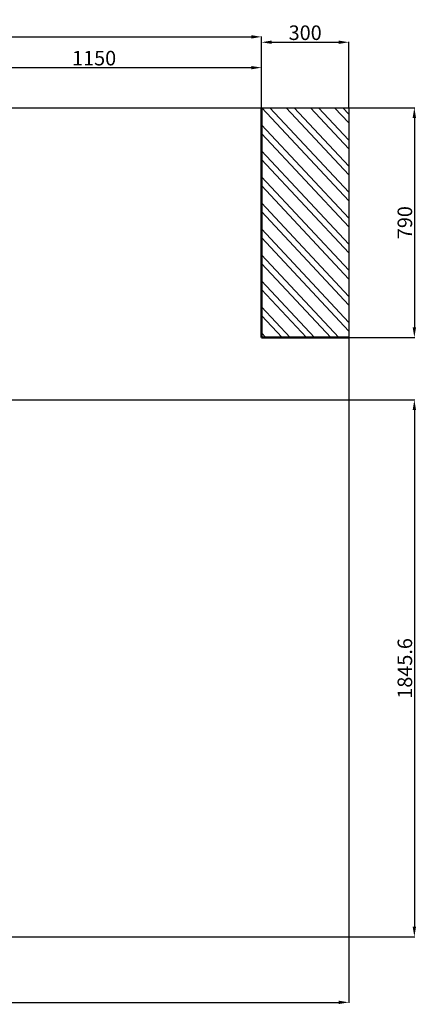
# Model space of a CAD drawing. Units: millimetres. Extents: x 407065 to 421840, y 1168257 to 1177792.
# Tile 2 of 17: x 410003 to 411365, y 1168454 to 1171838. Entities that reach past the tile are written whole.
import ezdxf

# ---------------------------------------------------------------- set-up
doc = ezdxf.new("R2010")
doc.units = ezdxf.units.MM
for name, color, linetype, lineweight in [('A-ANNO-DIMS', 6, 'Continuous', 18), ('A-FURN', 3, 'Continuous', 25), ('A-WALL', 7, 'Continuous', 50), ('A-WALL-PATT', 8, 'Continuous', 13)]:
    doc.layers.add(name, color=color, linetype=linetype, lineweight=lineweight)
doc.styles.get("Standard").update_dxf_attribs({"font": 'arial.ttf'})
doc.dimstyles.new('ISO-25', dxfattribs={"dimtxt": 50, "dimasz": 35, "dimexe": 1.25, "dimexo": 0.625, "dimtad": 1, "dimdec": 1, "dimtxsty": 'Standard', "dimcen": 35, "dimadec": 0, "dimazin": 0, "dimtfac": 1, "dimtdec": 1, "dimtmove": 0, "dimatfit": 3, "dimfxl": 1, "dimarcsym": 0})

# ---------------------------------------------------------------- blocks, each defined once
blk = doc.blocks.new('*D122')
at = {"layer": 'A-ANNO-DIMS', "color": 0, "lineweight": -2, "transparency": 16777216}
for p, q in [((409683.5, 1171673.4), (409683.5, 1171674.1)), ((409718.5, 1171672.8), (410798.5, 1171672.8)), ((410833.5, 1171673.4), (410833.5, 1171674.1))]:
    blk.add_line(p, q, dxfattribs=at)
at = {"layer": 'A-ANNO-DIMS', "color": 0, "transparency": 16777216}
for points in [[(409718.5, 1171678.6), (409718.5, 1171667), (409683.5, 1171672.8)], [(410798.5, 1171678.6), (410798.5, 1171667), (410833.5, 1171672.8)]]:
    blk.add_solid(points, dxfattribs=at)
at = {"layer": 'Defpoints', "color": 0, "transparency": 16777216}
for p in [(409683.5, 1171672.8), (410833.5, 1171672.8), (410833.5, 1171672.8)]:
    blk.add_point(p, dxfattribs=at)
at = {"layer": 'A-ANNO-DIMS', "color": 0, "transparency": 16777216, "insert": (410258.5, 1171699), "char_height": 50, "attachment_point": 5}
blk.add_mtext('1150', dxfattribs=at)
blk = doc.blocks.new('*D123')
at = {"layer": 'A-ANNO-DIMS', "color": 0, "lineweight": -2, "transparency": 16777216}
for p, q in [((408033.5, 1171744.1), (408033.5, 1171780)), ((408068.5, 1171778.7), (410798.5, 1171778.7)), ((410833.5, 1171744.1), (410833.5, 1171780))]:
    blk.add_line(p, q, dxfattribs=at)
at = {"layer": 'A-ANNO-DIMS', "color": 0, "transparency": 16777216}
for points in [[(408068.5, 1171784.5), (408068.5, 1171772.9), (408033.5, 1171778.7)], [(410798.5, 1171784.5), (410798.5, 1171772.9), (410833.5, 1171778.7)]]:
    blk.add_solid(points, dxfattribs=at)
at = {"layer": 'Defpoints', "color": 0, "transparency": 16777216}
for p in [(410833.5, 1171778.7), (408033.5, 1171743.5), (410833.5, 1171743.5)]:
    blk.add_point(p, dxfattribs=at)
at = {"layer": 'A-ANNO-DIMS', "color": 0, "transparency": 16777216, "insert": (409433.5, 1171804.9), "char_height": 50, "attachment_point": 5}
blk.add_mtext('2800', dxfattribs=at)
blk = doc.blocks.new('*D208')
at = {"layer": 'A-ANNO-DIMS', "color": 0, "lineweight": -2, "transparency": 16777216}
for p, q in [((407833.5, 1168684.6), (407833.5, 1168458.9)), ((411133.5, 1168684.6), (411133.5, 1168458.9)), ((407868.5, 1168460.2), (411098.5, 1168460.2))]:
    blk.add_line(p, q, dxfattribs=at)
at = {"layer": 'A-ANNO-DIMS', "color": 0, "transparency": 16777216}
for points in [[(407868.5, 1168466), (407868.5, 1168454.4), (407833.5, 1168460.2)], [(411098.5, 1168466), (411098.5, 1168454.4), (411133.5, 1168460.2)]]:
    blk.add_solid(points, dxfattribs=at)
at = {"layer": 'Defpoints', "color": 0, "transparency": 16777216}
for p in [(407833.5, 1168685.2), (411133.5, 1168685.2), (411133.5, 1168460.2)]:
    blk.add_point(p, dxfattribs=at)
at = {"layer": 'A-ANNO-DIMS', "color": 0, "transparency": 16777216, "insert": (409483.5, 1168486.4), "char_height": 50, "attachment_point": 5}
blk.add_mtext('3300', dxfattribs=at)
blk = doc.blocks.new('*D210')
at = {"layer": 'A-ANNO-DIMS', "color": 0, "lineweight": -2, "transparency": 16777216}
for p, q in [((410833.5, 1171535.8), (410833.5, 1171761.4)), ((410868.5, 1171760.2), (411098.5, 1171760.2)), ((411133.5, 1171535.8), (411133.5, 1171761.4))]:
    blk.add_line(p, q, dxfattribs=at)
at = {"layer": 'A-ANNO-DIMS', "color": 0, "transparency": 16777216}
for points in [[(410868.5, 1171766), (410868.5, 1171754.4), (410833.5, 1171760.2)], [(411098.5, 1171766), (411098.5, 1171754.4), (411133.5, 1171760.2)]]:
    blk.add_solid(points, dxfattribs=at)
at = {"layer": 'Defpoints', "color": 0, "transparency": 16777216}
for p in [(411133.5, 1171760.2), (410833.5, 1171535.2), (411133.5, 1171535.2)]:
    blk.add_point(p, dxfattribs=at)
at = {"layer": 'A-ANNO-DIMS', "color": 0, "transparency": 16777216, "insert": (410983.5, 1171786.4), "char_height": 50, "attachment_point": 5}
blk.add_mtext('300', dxfattribs=at)
blk = doc.blocks.new('*D211')
at = {"layer": 'A-ANNO-DIMS', "color": 0, "lineweight": -2, "transparency": 16777216}
for p, q in [((411134.2, 1171535.2), (411359.8, 1171535.2)), ((411358.5, 1171500.2), (411358.5, 1170780.2)), ((411134.2, 1170745.2), (411359.8, 1170745.2))]:
    blk.add_line(p, q, dxfattribs=at)
at = {"layer": 'A-ANNO-DIMS', "color": 0, "transparency": 16777216}
for points in [[(411352.7, 1171500.2), (411364.4, 1171500.2), (411358.5, 1171535.2)], [(411352.7, 1170780.2), (411364.4, 1170780.2), (411358.5, 1170745.2)]]:
    blk.add_solid(points, dxfattribs=at)
at = {"layer": 'Defpoints', "color": 0, "transparency": 16777216}
for p in [(411133.5, 1171535.2), (411133.5, 1170745.2), (411358.5, 1170745.2)]:
    blk.add_point(p, dxfattribs=at)
at = {"layer": 'A-ANNO-DIMS', "color": 0, "transparency": 16777216, "insert": (411332.4, 1171140.2), "char_height": 50, "attachment_point": 5, "rotation": 90}
blk.add_mtext('790', dxfattribs=at)
blk = doc.blocks.new('*D212')
at = {"layer": 'A-ANNO-DIMS', "color": 0, "lineweight": -2, "transparency": 16777216}
for p, q in [((409636.9, 1170530.8), (411359.8, 1170530.8)), ((411358.5, 1170495.8), (411358.5, 1168720.2)), ((409636.9, 1168685.2), (411359.8, 1168685.2))]:
    blk.add_line(p, q, dxfattribs=at)
at = {"layer": 'A-ANNO-DIMS', "color": 0, "transparency": 16777216}
for points in [[(411352.7, 1170495.8), (411364.4, 1170495.8), (411358.5, 1170530.8)], [(411352.7, 1168720.2), (411364.4, 1168720.2), (411358.5, 1168685.2)]]:
    blk.add_solid(points, dxfattribs=at)
at = {"layer": 'Defpoints', "color": 0, "transparency": 16777216}
for p in [(409636.3, 1170530.8), (409636.3, 1168685.2), (411358.5, 1168685.2)]:
    blk.add_point(p, dxfattribs=at)
at = {"layer": 'A-ANNO-DIMS', "color": 0, "transparency": 16777216, "insert": (411332.4, 1169608), "char_height": 50, "attachment_point": 5, "rotation": 90}
blk.add_mtext('1845.6', dxfattribs=at)

msp = doc.modelspace()

# ---------------------------------------------------------------- hatches: boundary and pattern name
at = {"layer": 'A-WALL-PATT'}
h = msp.add_hatch(dxfattribs=at)
h.set_pattern_fill('ANSI32', color=256, scale=6.4, angle=88)
h.set_pattern_definition([(133, (-5768.25, -464.17), (-44.5833217, -41.57462), []), (133, (-5767.245, -435.45), (-44.5833217, -41.57462), [])])
h.paths.add_polyline_path([(411133.5433, 1171535.1988), (410833.5433, 1171535.1988), (410833.5433, 1170745.1988), (411133.5433, 1170745.1988)])

# ---------------------------------------------------------------- linework, layer by layer
at = {"layer": 'A-FURN'}
for p, q in [((407833.5433, 1171535.1988), (411133.5433, 1171535.1988)), ((411133.5433, 1171535.1988), (411133.5433, 1168685.1988)), ((407833.5433, 1168685.1988), (411133.5433, 1168685.1988))]:
    msp.add_line(p, q, dxfattribs=at)
at = {"layer": 'A-WALL'}
for p, q in [((410833.5433, 1171535.1988), (410833.5433, 1170745.1988)), ((410833.5433, 1170745.1988), (411133.5433, 1170745.1988))]:
    msp.add_line(p, q, dxfattribs=at)

# ---------------------------------------------------------------- dimensions: what is measured, and where the dimension line sits
at = {"layer": 'A-ANNO-DIMS'}
for base, p1, p2, override, picture, middle in [((410833.5433, 1171778.705), (408033.5433, 1171743.4929), (410833.5433, 1171743.4929), {"dimclrd": 0, "dimclre": 0, "dimclrt": 0}, '*D123', (409433.5433, 1171804.8586)), ((411133.5433, 1171760.1988), (410833.5433, 1171535.1988), (411133.5433, 1171535.1988), {"dimdec": 0, "dimlfac": 1, "dimrnd": 0, "dimzin": 0, "dimdsep": 46, "dimlunit": 2}, '*D210', (410983.5433, 1171786.3695)), ((410833.5433, 1171672.8068), (409683.5433, 1171672.8068), (410833.5433, 1171672.8068), {"dimclrd": 0, "dimclre": 0, "dimclrt": 0}, '*D122', (410258.5433, 1171698.9605)), ((411133.5433, 1168460.1988), (407833.5433, 1168685.1988), (411133.5433, 1168685.1988), {"dimdec": 0, "dimlfac": 1, "dimrnd": 0, "dimzin": 0, "dimdsep": 46, "dimlunit": 2}, '*D208', (409483.5433, 1168486.3695))]:
    dim = msp.add_linear_dim(base=base, p1=p1, p2=p2, dimstyle='ISO-25', override=override, dxfattribs=at)
    dim.commit()
    dim.dimension.update_dxf_attribs({"geometry": picture, "text_midpoint": middle})
for base, p1, p2, override, picture, middle in [((411358.5433, 1170745.1988), (411133.5433, 1171535.1988), (411133.5433, 1170745.1988), {"dimdec": 0, "dimlfac": 1, "dimrnd": 0, "dimzin": 0, "dimdsep": 46, "dimlunit": 2}, '*D211', (411332.3896, 1171140.1988)), ((411358.5433, 1168685.1988), (409636.3246, 1170530.7673), (409636.3246, 1168685.1988), {"dimdec": 1, "dimlfac": 1, "dimrnd": 0, "dimzin": 0, "dimdsep": 46, "dimlunit": 2}, '*D212', (411332.3896, 1169607.9831))]:
    dim = msp.add_linear_dim(base=base, p1=p1, p2=p2, angle=90, dimstyle='ISO-25', override=override, dxfattribs=at)
    dim.commit()
    dim.dimension.update_dxf_attribs({"geometry": picture, "text_midpoint": middle})

doc.saveas('drawing.dxf')
